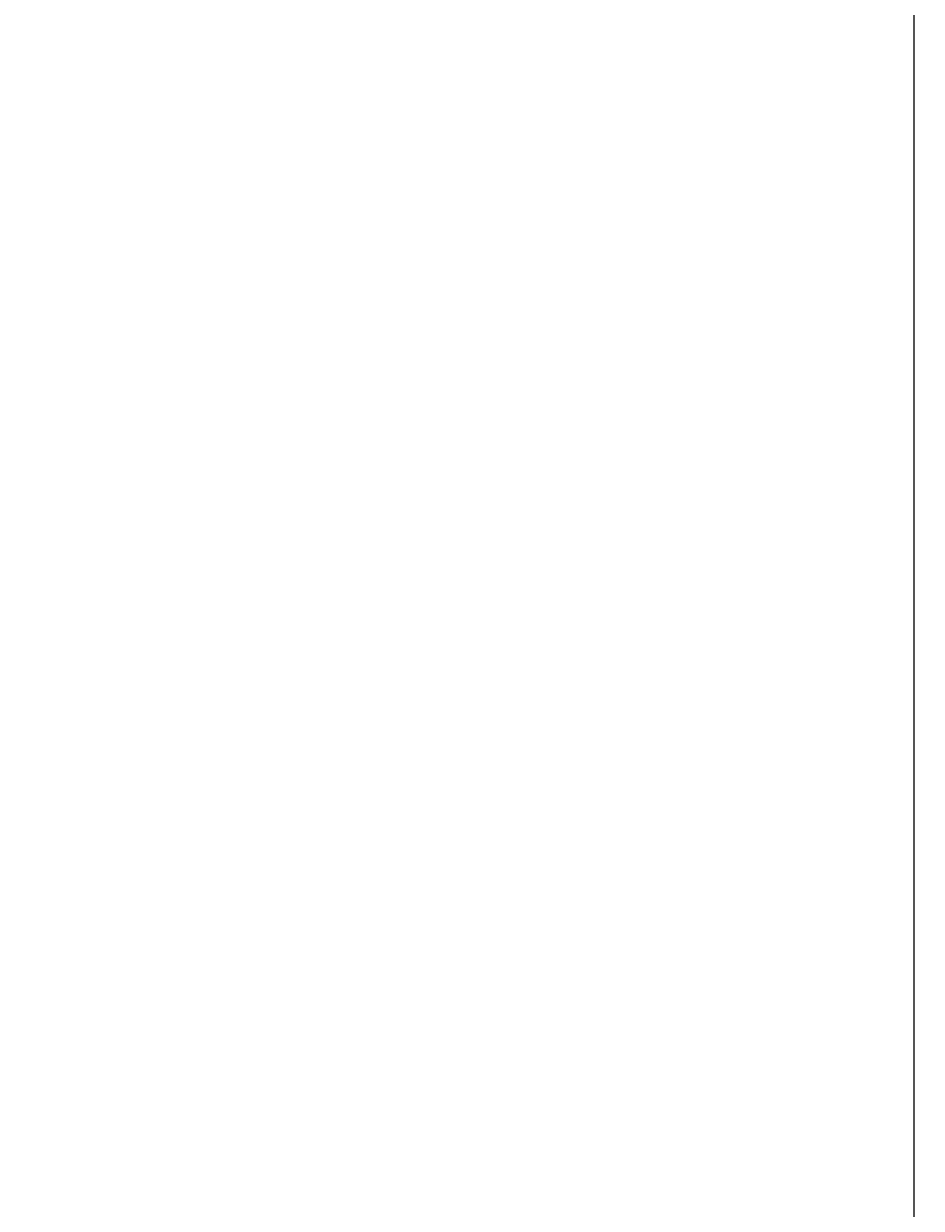
# Model space of a CAD drawing. Units: inches. Extents: x 1998 to 2588, y 1139 to 1977.
# Tile 112 of 134: x 2550 to 2588, y 1427 to 1477. Entities that reach past the tile are written whole.
import ezdxf

# ---------------------------------------------------------------- set-up
doc = ezdxf.new("R2010")
doc.units = ezdxf.units.IN
doc.layers.add('A-ANNO-DIMS', color=2, linetype='Continuous', lineweight=18)
doc.styles.get("Standard").update_dxf_attribs({"font": 'arial.ttf'})
doc.dimstyles.get("Standard").update_dxf_attribs({"dimtxt": 0.18, "dimasz": 0.18, "dimexe": 0.18, "dimexo": 0.0625, "dimgap": 0.09, "dimtad": 0, "dimtih": 1, "dimtoh": 1, "dimdec": 4, "dimzin": 0, "dimdsep": 46, "dimtxsty": 'Standard', "dimcen": 0.09, "dimadec": 0, "dimazin": 0, "dimtfac": 1, "dimtdec": 4, "dimtofl": 0, "dimtmove": 0, "dimatfit": 3, "dimfxl": 1, "dimtolj": 1, "dimtzin": 0, "dimarcsym": 0})

# ---------------------------------------------------------------- blocks, each defined once
blk = doc.blocks.new('*D24')
at = {"layer": 'A-ANNO-DIMS', "color": 0, "lineweight": -2, "transparency": 16777216}
for p, q in [((2398.535, 1911.232), (2588.309, 1911.232)), ((2588.129, 1911.052), (2588.129, 1570.164)), ((2588.129, 1228.912), (2588.129, 1569.8)), ((2527.535, 1228.732), (2588.309, 1228.732))]:
    blk.add_line(p, q, dxfattribs=at)
at = {"layer": 'A-ANNO-DIMS', "color": 0, "transparency": 16777216}
for points in [[(2588.099, 1911.052), (2588.159, 1911.052), (2588.129, 1911.232)], [(2588.099, 1228.912), (2588.159, 1228.912), (2588.129, 1228.732)]]:
    blk.add_solid(points, dxfattribs=at)
at = {"layer": 'Defpoints', "color": 0, "transparency": 16777216}
for p in [(2398.473, 1911.232), (2588.129, 1911.232), (2527.473, 1228.732)]:
    blk.add_point(p, dxfattribs=at)
at = {"layer": 'A-ANNO-DIMS', "color": 0, "transparency": 16777216, "insert": (2588.129, 1569.982), "char_height": 0.18, "attachment_point": 5}
blk.add_mtext('\\A1;682.5', dxfattribs=at)

msp = doc.modelspace()

# ---------------------------------------------------------------- dimensions: what is measured, and where the dimension line sits
at = {"layer": 'A-ANNO-DIMS'}
dim = msp.add_linear_dim(base=(2588.1286, 1911.2324), p1=(2527.4729, 1228.7324), p2=(2398.4729, 1911.2324), angle=90, dimstyle='Standard', override={"dimdec": 1, "dimlfac": 1, "dimrnd": 0, "dimzin": 0, "dimdsep": 46, "dimlunit": 2}, dxfattribs=at)
dim.commit()
dim.dimension.update_dxf_attribs({"geometry": '*D24', "text_midpoint": (2588.1286, 1569.9824)})

doc.saveas('drawing.dxf')
